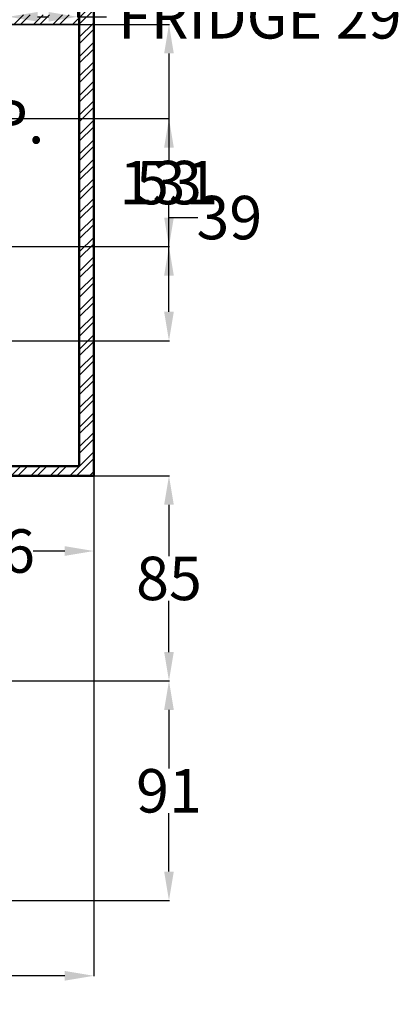
# Model space of a CAD drawing. Units: inches. Extents: x 7 to 752, y -275 to 426.
# Tile 4 of 5: x 596 to 752, y -271 to 137. Entities that reach past the tile are written whole.
import ezdxf

# ---------------------------------------------------------------- set-up
doc = ezdxf.new("R2010")
doc.units = ezdxf.units.IN
for name, color, linetype, lineweight in [('A-ANNO-DIMS', 2, 'Continuous', 18), ('A-WALL-PATT', 252, 'Continuous', 13), ('Inner Wall', 5, 'Continuous', 35), ('Outer Wall', 1, 'Continuous', 50)]:
    doc.layers.add(name, color=color, linetype=linetype, lineweight=lineweight)
doc.styles.get("Standard").update_dxf_attribs({"font": 'arial.ttf'})
doc.dimstyles.get("Standard").update_dxf_attribs({"dimtxt": 18, "dimasz": 12, "dimexe": 0.18, "dimexo": 0.0625, "dimgap": 0.09, "dimtad": 0, "dimtih": 1, "dimtoh": 1, "dimdec": 0, "dimzin": 0, "dimdsep": 46, "dimlunit": 3, "dimtxsty": 'Standard', "dimcen": 0.09, "dimadec": 0, "dimazin": 0, "dimtfac": 1, "dimtdec": 0, "dimtofl": 0, "dimtmove": 0, "dimatfit": 3, "dimfxl": 1, "dimtolj": 1, "dimtzin": 0, "dimarcsym": 0})
pattern_1 = [(45, (-434.707, -1257.0093), (-4.041115, 4.041115), []), (45, (-432.013, -1257.0093), (-4.041115, 4.041115), [])]

# ---------------------------------------------------------------- blocks, each defined once
blk = doc.blocks.new('*D20')
at = {"layer": 'A-ANNO-DIMS', "color": 0, "lineweight": -2, "transparency": 16777216}
for p, q in [((518.33, 134.68), (506.15, 134.68)), ((506.33, 122.68), (506.33, 103.84)), ((506.33, 66.2), (506.33, 85.04)), ((518.33, 54.2), (506.15, 54.2))]:
    blk.add_line(p, q, dxfattribs=at)
at = {"layer": 'A-ANNO-DIMS', "color": 0, "transparency": 16777216}
for points in [[(504.33, 122.68), (508.33, 122.68), (506.33, 134.68)], [(504.33, 66.2), (508.33, 66.2), (506.33, 54.2)]]:
    blk.add_solid(points, dxfattribs=at)
at = {"layer": 'Defpoints', "color": 0, "transparency": 16777216}
for p in [(506.33, 134.68), (518.4, 134.68), (518.4, 54.2)]:
    blk.add_point(p, dxfattribs=at)
at = {"layer": 'A-ANNO-DIMS', "color": 0, "transparency": 16777216, "insert": (506.33, 94.44), "char_height": 18, "attachment_point": 5}
blk.add_mtext('\\A1;KING BED 80 TYP.', dxfattribs=at)
blk = doc.blocks.new('*D26')
at = {"layer": 'A-ANNO-DIMS', "color": 0, "lineweight": -2, "transparency": 16777216}
for p, q in [((591.04, 142.1), (591.04, 137.69)), ((619.61, 142.1), (619.61, 137.69)), ((603.04, 137.87), (607.61, 137.87)), ((619.61, 137.87), (631.61, 137.87))]:
    blk.add_line(p, q, dxfattribs=at)
at = {"layer": 'A-ANNO-DIMS', "color": 0, "transparency": 16777216}
for points in [[(603.04, 139.87), (603.04, 135.87), (591.04, 137.87)], [(607.61, 139.87), (607.61, 135.87), (619.61, 137.87)]]:
    blk.add_solid(points, dxfattribs=at)
at = {"layer": 'Defpoints', "color": 0, "transparency": 16777216}
for p in [(591.04, 142.16), (619.61, 142.16), (619.61, 137.87)]:
    blk.add_point(p, dxfattribs=at)
at = {"layer": 'A-ANNO-DIMS', "color": 0, "transparency": 16777216, "insert": (695.1, 137.87), "char_height": 18, "attachment_point": 5}
blk.add_mtext('\\A1;FRIDGE 29', dxfattribs=at)
blk = doc.blocks.new('*D30')
at = {"layer": 'A-ANNO-DIMS', "color": 0, "lineweight": -2, "transparency": 16777216}
for p, q in [((626.33, -52.39), (626.33, -259.65)), ((158.33, -228.39), (158.33, -259.65)), ((170.33, -259.47), (371.97, -259.47)), ((614.33, -259.47), (412.68, -259.47))]:
    blk.add_line(p, q, dxfattribs=at)
at = {"layer": 'A-ANNO-DIMS', "color": 0, "transparency": 16777216}
for points in [[(170.33, -257.47), (170.33, -261.47), (158.33, -259.47)], [(614.33, -257.47), (614.33, -261.47), (626.33, -259.47)]]:
    blk.add_solid(points, dxfattribs=at)
at = {"layer": 'Defpoints', "color": 0, "transparency": 16777216}
for p in [(626.33, -52.32), (158.33, -228.32), (626.33, -259.47)]:
    blk.add_point(p, dxfattribs=at)
at = {"layer": 'A-ANNO-DIMS', "color": 0, "transparency": 16777216, "insert": (392.33, -259.47), "char_height": 18, "attachment_point": 5}
blk.add_mtext('\\A1;468', dxfattribs=at)
blk = doc.blocks.new('*D37')
at = {"layer": 'A-ANNO-DIMS', "color": 0, "lineweight": -2, "transparency": 16777216}
for p, q in [((626.39, -52.32), (657.66, -52.32)), ((657.48, -64.32), (657.48, -85.54)), ((657.48, -125.32), (657.48, -104.1)), ((550.39, -137.32), (657.66, -137.32))]:
    blk.add_line(p, q, dxfattribs=at)
at = {"layer": 'A-ANNO-DIMS', "color": 0, "transparency": 16777216}
for points in [[(655.48, -64.32), (659.48, -64.32), (657.48, -52.32)], [(655.48, -125.32), (659.48, -125.32), (657.48, -137.32)]]:
    blk.add_solid(points, dxfattribs=at)
at = {"layer": 'Defpoints', "color": 0, "transparency": 16777216}
for p in [(626.33, -52.32), (550.33, -137.32), (657.48, -137.32)]:
    blk.add_point(p, dxfattribs=at)
at = {"layer": 'A-ANNO-DIMS', "color": 0, "transparency": 16777216, "insert": (657.48, -94.82), "char_height": 18, "attachment_point": 5}
blk.add_mtext('\\A1;85', dxfattribs=at)
blk = doc.blocks.new('*D38')
at = {"layer": 'A-ANNO-DIMS', "color": 0, "lineweight": -2, "transparency": 16777216}
for p, q in [((550.39, -137.32), (657.66, -137.32)), ((657.48, -149.32), (657.48, -173.54)), ((657.48, -216.32), (657.48, -192.1)), ((360.39, -228.32), (657.66, -228.32))]:
    blk.add_line(p, q, dxfattribs=at)
at = {"layer": 'A-ANNO-DIMS', "color": 0, "transparency": 16777216}
for points in [[(655.48, -149.32), (659.48, -149.32), (657.48, -137.32)], [(655.48, -216.32), (659.48, -216.32), (657.48, -228.32)]]:
    blk.add_solid(points, dxfattribs=at)
at = {"layer": 'Defpoints', "color": 0, "transparency": 16777216}
for p in [(550.33, -137.32), (360.33, -228.32), (657.48, -228.32)]:
    blk.add_point(p, dxfattribs=at)
at = {"layer": 'A-ANNO-DIMS', "color": 0, "transparency": 16777216, "insert": (657.48, -182.82), "char_height": 18, "attachment_point": 5}
blk.add_mtext('\\A1;91', dxfattribs=at)
blk = doc.blocks.new('*D43')
at = {"layer": 'A-ANNO-DIMS', "color": 0, "lineweight": -2, "transparency": 16777216}
for p, q in [((221.39, 134.68), (657.66, 134.68)), ((657.48, 122.68), (657.48, 78.46)), ((657.48, 15.68), (657.48, 59.89)), ((221.39, 3.68), (657.66, 3.68))]:
    blk.add_line(p, q, dxfattribs=at)
at = {"layer": 'A-ANNO-DIMS', "color": 0, "transparency": 16777216}
for points in [[(655.48, 122.68), (659.48, 122.68), (657.48, 134.68)], [(655.48, 15.68), (659.48, 15.68), (657.48, 3.68)]]:
    blk.add_solid(points, dxfattribs=at)
at = {"layer": 'Defpoints', "color": 0, "transparency": 16777216}
for p in [(221.33, 134.68), (657.48, 134.68), (221.33, 3.68)]:
    blk.add_point(p, dxfattribs=at)
at = {"layer": 'A-ANNO-DIMS', "color": 0, "transparency": 16777216, "insert": (657.48, 69.18), "char_height": 18, "attachment_point": 5}
blk.add_mtext('\\A1;131', dxfattribs=at)
blk = doc.blocks.new('*D44')
at = {"layer": 'A-ANNO-DIMS', "color": 0, "lineweight": -2, "transparency": 16777216}
for p, q in [((657.48, 42.68), (657.48, 54.68)), ((657.48, 54.68), (669.48, 54.68)), ((284.39, 42.68), (657.66, 42.68)), ((657.48, 15.68), (657.48, 30.68)), ((284.39, 3.68), (657.66, 3.68))]:
    blk.add_line(p, q, dxfattribs=at)
at = {"layer": 'A-ANNO-DIMS', "color": 0, "transparency": 16777216}
for points in [[(655.48, 30.68), (659.48, 30.68), (657.48, 42.68)], [(655.48, 15.68), (659.48, 15.68), (657.48, 3.68)]]:
    blk.add_solid(points, dxfattribs=at)
at = {"layer": 'Defpoints', "color": 0, "transparency": 16777216}
for p in [(284.33, 42.68), (657.48, 42.68), (284.33, 3.68)]:
    blk.add_point(p, dxfattribs=at)
at = {"layer": 'A-ANNO-DIMS', "color": 0, "transparency": 16777216, "insert": (682.47, 54.68), "char_height": 18, "attachment_point": 5}
blk.add_mtext('\\A1;39', dxfattribs=at)
blk = doc.blocks.new('*D45')
at = {"layer": 'A-ANNO-DIMS', "color": 0, "lineweight": -2, "transparency": 16777216}
for p, q in [((284.39, 95.68), (657.66, 95.68)), ((657.48, 83.68), (657.48, 78.46)), ((657.48, 54.68), (657.48, 59.89)), ((284.39, 42.68), (657.66, 42.68))]:
    blk.add_line(p, q, dxfattribs=at)
at = {"layer": 'A-ANNO-DIMS', "color": 0, "transparency": 16777216}
for points in [[(655.48, 83.68), (659.48, 83.68), (657.48, 95.68)], [(655.48, 54.68), (659.48, 54.68), (657.48, 42.68)]]:
    blk.add_solid(points, dxfattribs=at)
at = {"layer": 'Defpoints', "color": 0, "transparency": 16777216}
for p in [(284.33, 95.68), (657.48, 95.68), (284.33, 42.68)]:
    blk.add_point(p, dxfattribs=at)
at = {"layer": 'A-ANNO-DIMS', "color": 0, "transparency": 16777216, "insert": (657.48, 69.18), "char_height": 18, "attachment_point": 5}
blk.add_mtext('\\A1;53', dxfattribs=at)
blk = doc.blocks.new('*D64')
at = {"layer": 'A-ANNO-DIMS', "color": 0, "lineweight": -2, "transparency": 16777216}
for p, q in [((550.33, -52.39), (550.33, -83.65)), ((626.33, -52.39), (626.33, -83.65)), ((562.33, -83.47), (575.43, -83.47)), ((614.33, -83.47), (601.23, -83.47))]:
    blk.add_line(p, q, dxfattribs=at)
at = {"layer": 'A-ANNO-DIMS', "color": 0, "transparency": 16777216}
for points in [[(562.33, -81.47), (562.33, -85.47), (550.33, -83.47)], [(614.33, -81.47), (614.33, -85.47), (626.33, -83.47)]]:
    blk.add_solid(points, dxfattribs=at)
at = {"layer": 'Defpoints', "color": 0, "transparency": 16777216}
for p in [(550.33, -52.32), (626.33, -52.32), (550.33, -83.47)]:
    blk.add_point(p, dxfattribs=at)
at = {"layer": 'A-ANNO-DIMS', "color": 0, "transparency": 16777216, "insert": (588.33, -83.47), "char_height": 18, "attachment_point": 5}
blk.add_mtext('\\A1;76', dxfattribs=at)

msp = doc.modelspace()

# ---------------------------------------------------------------- hatches: boundary and pattern name
at = {"layer": 'A-WALL-PATT'}
h = msp.add_hatch(dxfattribs=at)
h.set_pattern_fill('ANSI32', color=256, scale=0.6)
h.set_pattern_definition(pattern_1)
h.paths.add_polyline_path([(182.33, 376.68), (278.33, 376.68), (278.33, 306.68), (466.33, 306.68), (466.33, 312.68), (284.33, 312.68), (284.33, 382.68), (176.33, 382.68), (176.33, -48.32), (158.33, -48.32), (158.33, -228.32), (360.33, -228.32), (360.33, -137.32), (384.33, -137.32), (384.33, -131.32), (356.33, -131.32), (356.33, -222.32), (164.33, -222.32), (164.33, -54.32), (182.33, -54.32)])
h.paths.add_polyline_path([(626.33, 312.68), (502.33, 312.68), (502.33, 306.68), (620.33, 306.68), (620.33, 171.68), (620.33, -48.32), (544.33, -48.32), (544.33, -131.32), (432.33, -131.32), (432.33, -137.32), (550.33, -137.32), (550.33, -52.32), (626.33, -52.32)])
h = msp.add_hatch(dxfattribs=at)
h.set_pattern_fill('ANSI32', color=256, scale=0.6)
h.set_pattern_definition(pattern_1)
h.paths.add_polyline_path([(360.33, -48.32), (282.33, -48.32), (282.33, -44.32), (278.33, -44.32), (278.33, -48.32), (182.33, -48.32), (182.33, -54.32), (356.33, -54.32), (356.33, -89.32), (360.33, -89.32)])
h.paths.add_polyline_path([(484.33, -48.32), (460.33, -48.32), (460.33, -42.32), (456.33, -42.32), (456.33, -48.32), (432.33, -48.32), (432.33, -52.32), (456.33, -52.32), (456.33, -131.32), (460.33, -131.32), (460.33, -52.32), (484.33, -52.32)])
h.paths.add_polyline_path([(544.33, -48.32), (512.33, -48.32), (512.33, -52.32), (544.33, -52.32)])
h.paths.add_polyline_path([(460.33, 134.68), (484.33, 134.68), (620.33, 134.68), (620.33, 138.68), (460.33, 138.68), (460.33, 144.68), (456.33, 144.68), (456.33, -6.32), (460.33, -6.32)])
h.paths.add_polyline_path([(282.33, 3.68), (182.33, 3.68), (182.33, -0.32), (278.33, -0.32), (278.33, -16.32), (282.33, -16.32)])
h.paths.add_polyline_path([(378.33, 144.68), (374.33, 144.68), (374.33, 138.68), (182.33, 138.68), (182.33, 134.68), (378.33, 134.68)])
h.paths.add_polyline_path([(284.33, 306.68), (278.33, 306.68), (278.33, 286.68), (240.33, 286.68), (240.33, 282.68), (284.33, 282.68)])
h.paths.add_polyline_path([(212.33, 286.68), (182.33, 286.68), (182.33, 282.68), (212.33, 282.68)])
h.paths.add_polyline_path([(436.33, 225.08), (460.33, 225.08), (460.33, 229.08), (432.33, 229.08), (432.33, 184.68), (456.33, 184.68), (456.33, 180.68), (460.33, 180.68), (460.33, 188.68), (436.33, 188.68)])
h.paths.add_polyline_path([(432.33, 204.68), (378.33, 204.68), (378.33, 306.68), (374.33, 306.68), (374.33, 282.68), (374.33, 198.85), (374.33, 180.68), (378.33, 180.68), (378.33, 200.68), (432.33, 200.68)])
h.paths.add_polyline_path([(460.33, 270.68), (436.33, 270.68), (436.33, 306.68), (432.33, 306.68), (432.33, 282.68), (432.33, 266.68), (460.33, 266.68)])

# ---------------------------------------------------------------- linework, layer by layer
at = {"layer": 'Inner Wall'}
msp.add_line((460.33, 134.68), (620.33, 134.68), dxfattribs=at)
at = {"layer": 'Outer Wall'}
for p, q in [((626.33, -52.32), (626.33, 312.68)), ((620.33, -48.32), (620.33, 306.68)), ((544.33, -48.32), (620.33, -48.32)), ((550.33, -52.32), (626.33, -52.32))]:
    msp.add_line(p, q, dxfattribs=at)

# ---------------------------------------------------------------- dimensions: what is measured, and where the dimension line sits
at = {"layer": 'A-ANNO-DIMS'}
dim = msp.add_linear_dim(base=(619.61, 137.87), p1=(591.04, 142.16), p2=(619.61, 142.16), text='FRIDGE <>', dimstyle='Standard', override={"dimdec": 0, "dimlfac": 1, "dimrnd": 0, "dimzin": 0, "dimdsep": 46, "dimlunit": 2}, dxfattribs=at)
dim.commit()
dim.dimension.update_dxf_attribs({"geometry": '*D26', "text_midpoint": (695.1, 137.87)})
dim = msp.add_linear_dim(base=(506.33, 134.68), p1=(518.4, 54.2), p2=(518.4, 134.68), angle=90, text='KING BED <> TYP.', dimstyle='Standard', override={"dimdec": 0, "dimlfac": 1, "dimrnd": 0, "dimzin": 0, "dimdsep": 46, "dimlunit": 2}, dxfattribs=at)
dim.commit()
dim.dimension.update_dxf_attribs({"geometry": '*D20', "text_midpoint": (506.33, 94.44)})
for base, p1, p2, angle, picture, middle in [((657.48, 134.68), (221.33, 3.68), (221.33, 134.68), 90, '*D43', (657.48, 69.18)), ((657.48, 95.68), (284.33, 42.68), (284.33, 95.68), 90, '*D45', (657.48, 69.18)), ((657.48, 42.68), (284.33, 3.68), (284.33, 42.68), 90, '*D44', (682.47, 54.68)), ((657.48, -137.32), (626.33, -52.32), (550.33, -137.32), 90, '*D37', (657.48, -94.82)), ((550.33, -83.47), (626.33, -52.32), (550.33, -52.32), 180, '*D64', (588.33, -83.47)), ((657.48, -228.32), (550.33, -137.32), (360.33, -228.32), 90, '*D38', (657.48, -182.82))]:
    dim = msp.add_linear_dim(base=base, p1=p1, p2=p2, angle=angle, dimstyle='Standard', override={"dimdec": 0, "dimlfac": 1, "dimrnd": 0, "dimzin": 0, "dimdsep": 46, "dimlunit": 2}, dxfattribs=at)
    dim.commit()
    dim.dimension.update_dxf_attribs({"geometry": picture, "text_midpoint": middle})
dim = msp.add_linear_dim(base=(626.33, -259.47), p1=(158.33, -228.32), p2=(626.33, -52.32), dimstyle='Standard', override={"dimdec": 0, "dimlfac": 1, "dimrnd": 0, "dimzin": 0, "dimdsep": 46, "dimlunit": 2}, dxfattribs=at)
dim.commit()
dim.dimension.update_dxf_attribs({"geometry": '*D30', "text_midpoint": (392.33, -259.47)})

doc.saveas('drawing.dxf')
